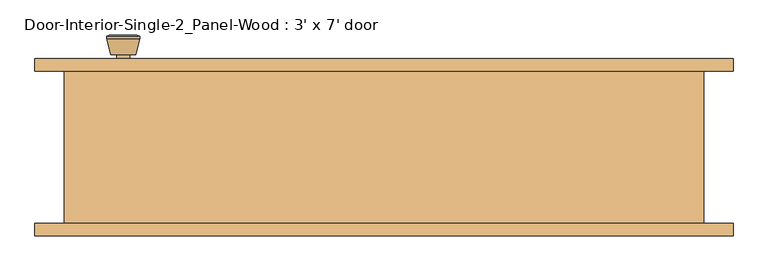
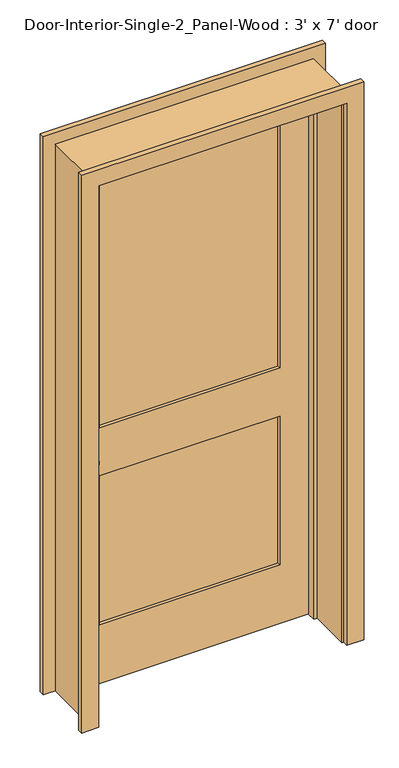
"""IFC4 building model written with IfcOpenShell, lengths in millimetres: door geometry, Door-Interior-Single-2_Panel-Wood : 3' x 7' door."""

from ifc_helpers import new_model, si_unit, point, frame, frame_2d, origin, place, context, project, spatial, polyline, circle_curve, trimmed, segment, composite_curve, outline, extrude, faceted_brep, source, transform, mapped, element, save
from ifc_brep_helpers import plane_surface, cylinder_surface, revolved_surface, advanced_brep


def door_interior_single_2_panel_wood_3_x_7_door_08fe406f(model_context):
    return source(origin(), model_context, "Body", "SolidModel", [
        advanced_brep(
        [(-393.7, 70.9, 914.4), (-383.7, 70.9, 914.4), (-403.7, 70.9, 914.4), (-373.2241324, 21.9, 914.4), (-393.7, 21.9, 914.4), (-414.1758676, 21.9, 914.4), (-368.7, 23.7278681, 914.4), (-418.7, 23.7278681, 914.4), (-368.7, 27.1915463, 914.4), (-418.7, 27.1915463, 914.4), (-375.063764, 51.9, 914.4), (-412.336236, 51.9, 914.4), (-383.7, 51.9, 914.4), (-403.7, 51.9, 914.4)],
        [
            (0, 1),
            (1, 2, circle_curve(frame((-393.7, 70.9, 914.4), z_axis=(0.0, 1.0, 0.0), x_axis=(-1.0, 0.0, 0.0)), 10.0)),
            (2, 0),
            (2, 1, circle_curve(frame((-393.7, 70.9, 914.4), z_axis=(0.0, 1.0, 0.0), x_axis=(-1.0, 0.0, 0.0)), 10.0)),
            (3, 4),
            (4, 5),
            (5, 3, circle_curve(frame((-393.7, 21.9, 914.4), z_axis=(0.0, -1.0, 0.0), x_axis=(-1.0, 0.0, 0.0)), 20.4758676)),
            (3, 5, circle_curve(frame((-393.7, 21.9, 914.4), z_axis=(0.0, -1.0, 0.0), x_axis=(-1.0, 0.0, 0.0)), 20.4758676)),
            (6, 3),
            (5, 7),
            (7, 6, circle_curve(frame((-393.7, 23.7278681, 914.4), z_axis=(0.0, -1.0, 0.0), x_axis=(-1.0, 0.0, 0.0)), 25.0)),
            (6, 7, circle_curve(frame((-393.7, 23.7278681, 914.4), z_axis=(0.0, -1.0, 0.0), x_axis=(-1.0, 0.0, 0.0)), 25.0)),
            (8, 6),
            (7, 9),
            (9, 8, circle_curve(frame((-393.7, 27.1915463, 914.4), z_axis=(0.0, -1.0, 0.0), x_axis=(-1.0, 0.0, 0.0)), 25.0)),
            (8, 9, circle_curve(frame((-393.7, 27.1915463, 914.4), z_axis=(0.0, -1.0, 0.0), x_axis=(-1.0, 0.0, 0.0)), 25.0)),
            (10, 8),
            (9, 11),
            (11, 10, circle_curve(frame((-393.7, 51.9, 914.4), z_axis=(0.0, -1.0, 0.0), x_axis=(-1.0, 0.0, 0.0)), 18.636236)),
            (10, 11, circle_curve(frame((-393.7, 51.9, 914.4), z_axis=(0.0, -1.0, 0.0), x_axis=(-1.0, 0.0, 0.0)), 18.636236)),
            (12, 10),
            (11, 13),
            (13, 12, circle_curve(frame((-393.7, 51.9, 914.4), z_axis=(0.0, -1.0, 0.0), x_axis=(-1.0, 0.0, 0.0)), 10.0)),
            (12, 13, circle_curve(frame((-393.7, 51.9, 914.4), z_axis=(0.0, -1.0, 0.0), x_axis=(-1.0, 0.0, 0.0)), 10.0)),
            (1, 12),
            (13, 2),
        ],
        [
            plane_surface(frame((-393.7, 70.9, 914.4), z_axis=(0.0, 1.0, 0.0), x_axis=(-1.0, 0.0, 0.0))),
            plane_surface(frame((-393.7, 21.9, 914.4), z_axis=(0.0, -1.0, 0.0), x_axis=(-1.0, 0.0, 0.0))),
            revolved_surface(polyline([(-414.1758676, 21.9, 914.4), (-418.7, 23.7278681, 914.4)]), (-393.7, 70.9, 914.4), (0.0, 1.0, 0.0)),
            cylinder_surface(frame((-393.7, 70.9, 914.4), z_axis=(0.0, 1.0, 0.0), x_axis=(-1.0, 0.0, 0.0)), 25.0),
            revolved_surface(polyline([(-418.7, 27.1915463, 914.4), (-412.336236, 51.9, 914.4)]), (-393.7, 70.9, 914.4), (0.0, 1.0, 0.0)),
            plane_surface(frame((-393.7, 51.9, 914.4), z_axis=(0.0, 1.0, 0.0), x_axis=(-1.0, 0.0, 0.0))),
            cylinder_surface(frame((-393.7, 70.9, 914.4), z_axis=(0.0, 1.0, 0.0), x_axis=(-1.0, 0.0, 0.0)), 10.0),
        ],
        [
            (0, [[1, 2, 3]]),
            (0, [[-3, 4, -1]]),
            (1, [[5, 6, 7]]),
            (1, [[-6, -5, 8]]),
            (2, [[9, -7, 10, 11]]),
            (2, [[-10, -8, -9, 12]]),
            (3, [[13, -11, 14, 15]]),
            (3, [[-14, -12, -13, 16]]),
            (4, [[17, -15, 18, 19]]),
            (4, [[-18, -16, -17, 20]]),
            (5, [[21, -19, 22, 23]]),
            (5, [[-22, -20, -21, 24]]),
            (6, [[25, -23, 26, -2]]),
            (6, [[-26, -24, -25, -4]]),
        ],
    ),
        extrude(outline(composite_curve([segment(trimmed(circle_curve(frame_2d((914.4, -393.7)), 30.0), [point((914.4, -423.7))], [point((914.4, -363.7))], False, "CARTESIAN"), True, "CONTINUOUS"), segment(trimmed(circle_curve(frame_2d((914.4, -393.7)), 30.0), [point((914.4, -363.7))], [point((914.4, -423.7))], False, "CARTESIAN"), True, "CONTINUOUS")], self_intersect=False)), frame((0.0, 70.9, 0.0), z_axis=(0.0, 1.0, 0.0), x_axis=(0.0, 0.0, 1.0)), (0.0, 0.0, 1.0), 6.0),
        advanced_brep(
        [(-393.7, 117.825, 914.4), (-403.7, 117.825, 914.4), (-383.7, 117.825, 914.4), (-373.2241324, 166.825, 914.4), (-414.1758676, 166.825, 914.4), (-393.7, 166.825, 914.4), (-368.7, 164.9971319, 914.4), (-418.7, 164.9971319, 914.4), (-368.7, 161.5334537, 914.4), (-418.7, 161.5334537, 914.4), (-375.063764, 136.825, 914.4), (-412.336236, 136.825, 914.4), (-383.7, 136.825, 914.4), (-403.7, 136.825, 914.4)],
        [
            (0, 1),
            (1, 2, circle_curve(frame((-393.7, 117.825, 914.4), z_axis=(0.0, -1.0, 0.0), x_axis=(-1.0, 0.0, 0.0)), 10.0)),
            (2, 0),
            (2, 1, circle_curve(frame((-393.7, 117.825, 914.4), z_axis=(0.0, -1.0, 0.0), x_axis=(-1.0, 0.0, 0.0)), 10.0)),
            (3, 4, circle_curve(frame((-393.7, 166.825, 914.4), z_axis=(0.0, 1.0, 0.0), x_axis=(-1.0, 0.0, 0.0)), 20.4758676)),
            (4, 5),
            (5, 3),
            (4, 3, circle_curve(frame((-393.7, 166.825, 914.4), z_axis=(0.0, 1.0, 0.0), x_axis=(-1.0, 0.0, 0.0)), 20.4758676)),
            (6, 7, circle_curve(frame((-393.7, 164.9971319, 914.4), z_axis=(0.0, 1.0, 0.0), x_axis=(-1.0, 0.0, 0.0)), 25.0)),
            (7, 4),
            (3, 6),
            (7, 6, circle_curve(frame((-393.7, 164.9971319, 914.4), z_axis=(0.0, 1.0, 0.0), x_axis=(-1.0, 0.0, 0.0)), 25.0)),
            (8, 9, circle_curve(frame((-393.7, 161.5334537, 914.4), z_axis=(0.0, 1.0, 0.0), x_axis=(-1.0, 0.0, 0.0)), 25.0)),
            (9, 7),
            (6, 8),
            (9, 8, circle_curve(frame((-393.7, 161.5334537, 914.4), z_axis=(0.0, 1.0, 0.0), x_axis=(-1.0, 0.0, 0.0)), 25.0)),
            (10, 11, circle_curve(frame((-393.7, 136.825, 914.4), z_axis=(0.0, 1.0, 0.0), x_axis=(-1.0, 0.0, 0.0)), 18.636236)),
            (11, 9),
            (8, 10),
            (11, 10, circle_curve(frame((-393.7, 136.825, 914.4), z_axis=(0.0, 1.0, 0.0), x_axis=(-1.0, 0.0, 0.0)), 18.636236)),
            (12, 13, circle_curve(frame((-393.7, 136.825, 914.4), z_axis=(0.0, 1.0, 0.0), x_axis=(-1.0, 0.0, 0.0)), 10.0)),
            (13, 11),
            (10, 12),
            (13, 12, circle_curve(frame((-393.7, 136.825, 914.4), z_axis=(0.0, 1.0, 0.0), x_axis=(-1.0, 0.0, 0.0)), 10.0)),
            (1, 13),
            (12, 2),
        ],
        [
            plane_surface(frame((-393.7, 117.825, 914.4), z_axis=(0.0, -1.0, 0.0), x_axis=(-1.0, 0.0, 0.0))),
            plane_surface(frame((-393.7, 166.825, 914.4), z_axis=(0.0, 1.0, 0.0), x_axis=(-1.0, 0.0, 0.0))),
            revolved_surface(polyline([(-414.1758676, 166.825, 914.4), (-418.7, 164.9971319, 914.4)]), (-393.7, 117.825, 914.4), (0.0, -1.0, 0.0)),
            cylinder_surface(frame((-393.7, 117.825, 914.4), z_axis=(0.0, -1.0, 0.0), x_axis=(-1.0, 0.0, 0.0)), 25.0),
            revolved_surface(polyline([(-418.7, 161.5334537, 914.4), (-412.336236, 136.825, 914.4)]), (-393.7, 117.825, 914.4), (0.0, -1.0, 0.0)),
            plane_surface(frame((-393.7, 136.825, 914.4), z_axis=(0.0, -1.0, 0.0), x_axis=(-1.0, 0.0, 0.0))),
            cylinder_surface(frame((-393.7, 117.825, 914.4), z_axis=(0.0, -1.0, 0.0), x_axis=(-1.0, 0.0, 0.0)), 10.0),
        ],
        [
            (0, [[1, 2, 3]]),
            (0, [[-3, 4, -1]]),
            (1, [[5, 6, 7]]),
            (1, [[8, -7, -6]]),
            (2, [[9, 10, -5, 11]]),
            (2, [[12, -11, -8, -10]]),
            (3, [[13, 14, -9, 15]]),
            (3, [[16, -15, -12, -14]]),
            (4, [[17, 18, -13, 19]]),
            (4, [[20, -19, -16, -18]]),
            (5, [[21, 22, -17, 23]]),
            (5, [[24, -23, -20, -22]]),
            (6, [[-2, 25, -21, 26]]),
            (6, [[-4, -26, -24, -25]]),
        ],
    ),
        extrude(outline(composite_curve([segment(trimmed(circle_curve(frame_2d((914.4, -393.7)), 30.0), [point((914.4, -423.7))], [point((914.4, -363.7))], False, "CARTESIAN"), True, "CONTINUOUS"), segment(trimmed(circle_curve(frame_2d((914.4, -393.7)), 30.0), [point((914.4, -363.7))], [point((914.4, -423.7))], False, "CARTESIAN"), True, "CONTINUOUS")], self_intersect=False)), frame((0.0, 111.825, 0.0), z_axis=(0.0, 1.0, 0.0), x_axis=(0.0, 0.0, 1.0)), (0.0, 0.0, 1.0), 6.0),
        faceted_brep([(482.6, 111.825, 0.0), (482.6, -118.175, 0.0), (457.2, -118.175, 0.0), (457.2, 41.975, 0.0), (444.5, 41.975, 0.0), (444.5, 76.9, 0.0), (457.2, 76.9, 0.0), (457.2, 111.825, 0.0), (482.6, 111.825, 2159.0), (482.6, -118.175, 2159.0), (-482.6, -118.175, 2159.0), (-482.6, -118.175, 0.0), (-457.2, -118.175, 0.0), (-457.2, -118.175, 2133.6), (457.2, -118.175, 2133.6), (457.2, 41.975, 2133.6), (-457.2, 41.975, 2133.6), (-457.2, 41.975, 0.0), (-444.5, 41.975, 0.0), (-444.5, 41.975, 2120.9), (444.5, 41.975, 2120.9), (444.5, 76.9, 2120.9), (-444.5, 76.9, 2120.9), (-444.5, 76.9, 0.0), (-457.2, 76.9, 0.0), (-457.2, 76.9, 2133.6), (457.2, 76.9, 2133.6), (457.2, 111.825, 2133.6), (-457.2, 111.825, 2133.6), (-457.2, 111.825, 0.0), (-482.6, 111.825, 0.0), (-482.6, 111.825, 2159.0)], [[[0, 1, 2, 3, 4, 5, 6, 7]], [[1, 0, 8, 9]], [[2, 1, 9, 10, 11, 12, 13, 14]], [[3, 2, 14, 15]], [[4, 3, 15, 16, 17, 18, 19, 20]], [[5, 4, 20, 21]], [[6, 5, 21, 22, 23, 24, 25, 26]], [[7, 6, 26, 27]], [[0, 7, 27, 28, 29, 30, 31, 8]], [[9, 8, 31, 10]], [[15, 14, 13, 16]], [[21, 20, 19, 22]], [[27, 26, 25, 28]], [[30, 29, 24, 23, 18, 17, 12, 11]], [[10, 31, 30, 11]], [[16, 13, 12, 17]], [[22, 19, 18, 23]], [[28, 25, 24, 29]]]),
        extrude(outline(polyline([(2133.6, -457.2), (0.0, -457.2), (0.0, 457.2), (2133.6, 457.2), (2133.6, -457.2)]), holes=[polyline([(2014.5375, -336.55), (2014.5375, 336.55), (1009.65, 336.55), (1009.65, -336.55), (2014.5375, -336.55)]), polyline([(819.15, -336.55), (819.15, 336.55), (231.775, 336.55), (231.775, -336.55), (819.15, -336.55)])]), frame((0.0, 76.9, 0.0), z_axis=(0.0, 1.0, 0.0), x_axis=(0.0, 0.0, 1.0)), (0.0, 0.0, 1.0), 34.925),
        extrude(outline(polyline([(336.55, 88.5416667), (-336.55, 88.5416667), (-336.55, 100.1833333), (336.55, 100.1833333), (336.55, 88.5416667)])), frame((0.0, 0.0, 1009.65), z_axis=(0.0, 0.0, 1.0), x_axis=(1.0, 0.0, 0.0)), (0.0, 0.0, 1.0), 1004.8875),
        extrude(outline(polyline([(336.55, 88.5416667), (-336.55, 88.5416667), (-336.55, 100.1833333), (336.55, 100.1833333), (336.55, 88.5416667)])), frame((0.0, 0.0, 231.775), z_axis=(0.0, 0.0, 1.0), x_axis=(1.0, 0.0, 0.0)), (0.0, 0.0, 1.0), 587.375),
        extrude(outline(polyline([(0.0, 463.55), (0.0, 527.05), (2203.45, 527.05), (2203.45, -527.05), (0.0, -527.05), (0.0, -463.55), (2139.95, -463.55), (2139.95, 463.55), (0.0, 463.55)])), frame((0.0, 111.825, 0.0), z_axis=(0.0, 1.0, 0.0), x_axis=(0.0, 0.0, 1.0)), (0.0, 0.0, 1.0), 19.05),
        extrude(outline(polyline([(0.0, 463.55), (0.0, 527.05), (2203.45, 527.05), (2203.45, -527.05), (0.0, -527.05), (0.0, -463.55), (2139.95, -463.55), (2139.95, 463.55), (0.0, 463.55)])), frame((0.0, -137.225, 0.0), z_axis=(0.0, 1.0, 0.0), x_axis=(0.0, 0.0, 1.0)), (0.0, 0.0, 1.0), 19.05),
    ])


if __name__ == "__main__":
    model = new_model("IFC4")
    model_context = context("Model", 3, world=origin())
    ifc_project = project(units=[si_unit("LENGTHUNIT", "METRE", prefix="MILLI")], contexts=[model_context])
    site = spatial("IfcSite", under=ifc_project)
    building = spatial("IfcBuilding", under=site)
    placement = place(None, origin())
    door_interior_single_2_panel_wood_3_x_7_door_shape = door_interior_single_2_panel_wood_3_x_7_door_08fe406f(model_context)
    element("IfcDoor", 1, ObjectType="Door-Interior-Single-2_Panel-Wood : 3' x 7' door", at=placement, inside=building, context=model_context, shape_type="MappedRepresentation", body=[
        mapped(door_interior_single_2_panel_wood_3_x_7_door_shape, transform((0.0, 0.0, 0.0), x_axis=(1.0, 0.0, 0.0), y_axis=(0.0, 1.0, 0.0), z_axis=(0.0, 0.0, 1.0))),
    ])
    save(model, "model.ifc")

# Revit data of these elements
# Type "Door-Interior-Single-2_Panel-Wood : 3' x 7' door"
#   Type Mark = "9"
#   Assembly Code = "C1020300"
#   Analytic Construction = "Wooden"
#   Top Rail = 0' - 4 11/16"
#   Thickness = 0' - 1 3/8"
#   Thermal Resistance (R) = 2.5876 (h·ft²·°F)/BTU
#   Swing Angle [instance default] = 90.00°
#   Stiles = 0' - 4 3/4"
#   Rough Width = 3' - 2"
#   Rough Height = 7' - 1"
#   Lock Rail = 0' - 7 1/2"
#   Height = 7' - 0"
#   Width = 3' - 0"
#   Heat Transfer Coefficient (U) = 0.3865 BTU/(h·ft²·°F)
#   Bottom Rail = 0' - 9 1/8"
#   Trim Material = Cherry
#   Panel Material = Cherry
#   Frame Material = Cherry
#   Door Handle Material = Aluminum
#   Visual Light Transmittance = 0
#   Solar Heat Gain Coefficient = 0
#   Wall Closure = (empty or 0)
#   Function = (empty or 0)
# Element 1 (IfcDoor, "Door-Interior-Single-2_Panel-Wood : 3' x 7' door")
#   Materials on its faces: "Cherry", "Aluminum"
# Materials
#   "Cherry": class "Wood", colour RGB 226 177 128, transparency 0, Description = "Prunus Serotina", Cost = 0
#   "Aluminum": class "Metal", colour RGB 247 247 247, transparency 0, Description = "Aluminum 6061", Cost = 0
